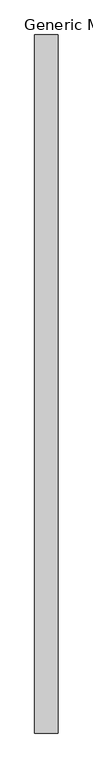
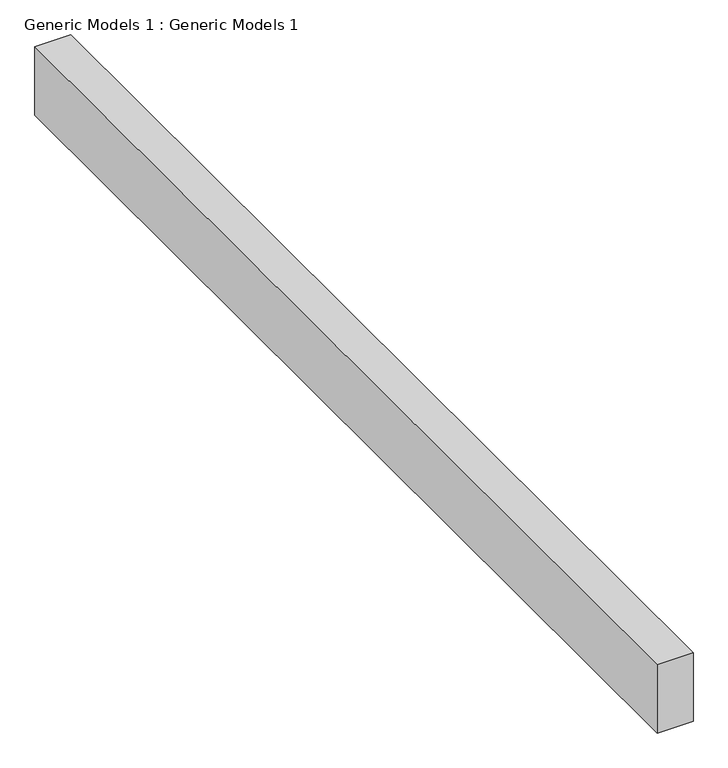
"""IFC4 building model written with IfcOpenShell, lengths in millimetres: proxy geometry, Generic Models 1 : Generic Models 1."""

from ifc_helpers import new_model, si_unit, frame, origin, place, context, project, spatial, polyline, outline, extrude, source, transform, mapped, element, save


def generic_models_1_generic_models_1_af82f8a7(model_context):
    return source(origin(), model_context, "Body", "SweptSolid", [
        extrude(outline(polyline([(4494.3719693, 9279.7858582), (4494.3719693, 165.8100141), (4189.5719693, 165.8100141), (4189.5719693, 9279.7858582), (4494.3719693, 9279.7858582)])), frame((0.0, 0.0, 3035.79831), z_axis=(0.0, 0.0, 1.0), x_axis=(1.0, 0.0, 0.0)), (0.0, 0.0, 1.0), 609.6),
    ])


if __name__ == "__main__":
    model = new_model("IFC4")
    model_context = context("Model", 3, world=origin())
    ifc_project = project(units=[si_unit("LENGTHUNIT", "METRE", prefix="MILLI")], contexts=[model_context])
    site = spatial("IfcSite", under=ifc_project)
    building = spatial("IfcBuilding", under=site)
    placement = place(None, origin())
    generic_models_1_generic_models_1_shape = generic_models_1_generic_models_1_af82f8a7(model_context)
    element("IfcBuildingElementProxy", 1, Name="Generic Models 1 : Generic Models 1", ObjectType="Generic Models 1 : Generic Models 1", at=placement, inside=building, context=model_context, shape_type="MappedRepresentation", body=[
        mapped(generic_models_1_generic_models_1_shape, transform((0.0, 0.0, 0.0), x_axis=(1.0, 0.0, 0.0), y_axis=(0.0, 1.0, 0.0), z_axis=(0.0, 0.0, 1.0))),
    ])
    save(model, "model.ifc")

# Revit data of these elements
# Element 1 (IfcBuildingElementProxy, "Generic Models 1 : Generic Models 1")
#   Materials on its faces: "OUTER WALL 9\""
# Materials
#   "OUTER WALL 9\"": class "Generic", colour RGB 120 120 120, transparency 0, Cost = 0
